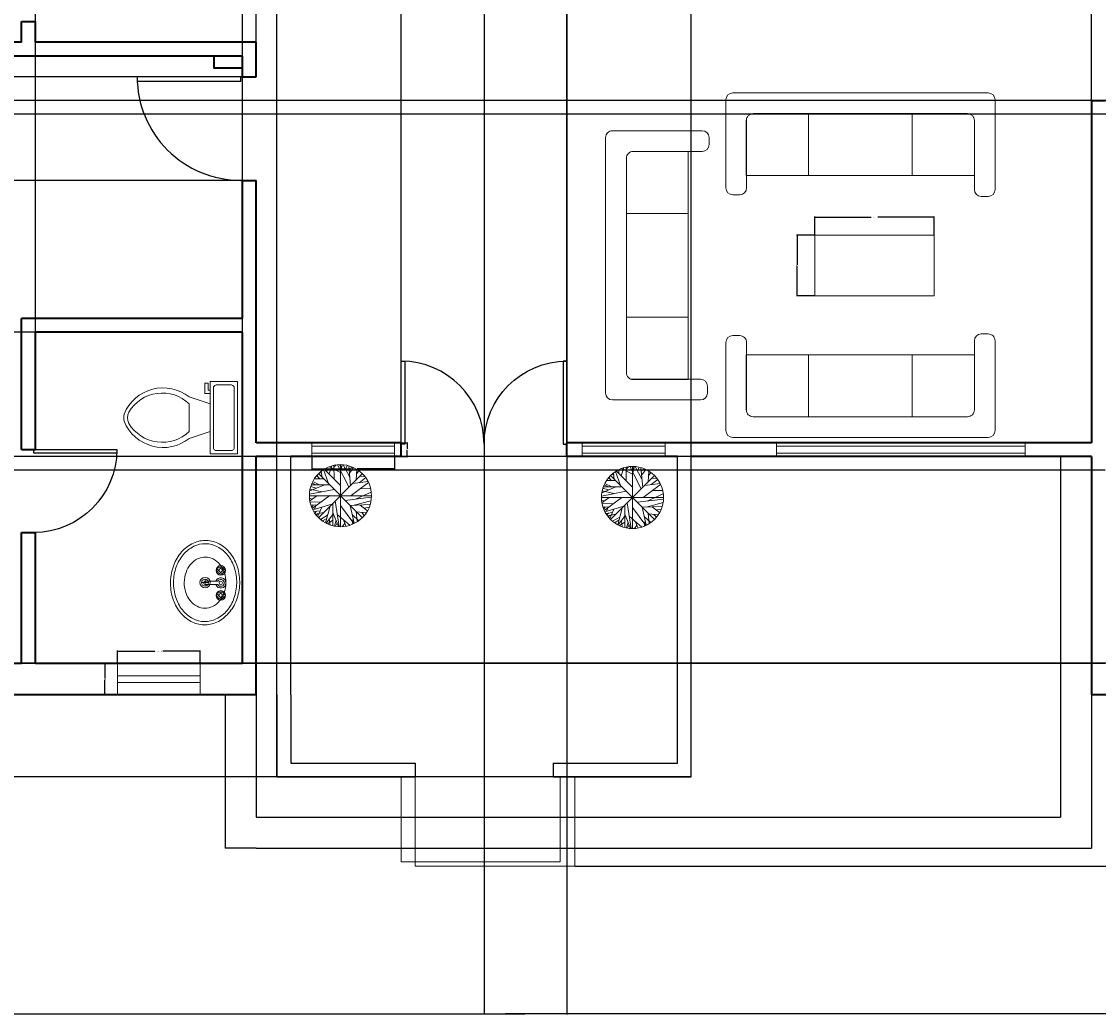
# Model space of a CAD drawing. Units: inches. Extents: x 2024 to 2965, y 1692 to 2308.
# Tile 4 of 8: x 2355 to 2667, y 1692 to 1980. Entities that reach past the tile are written whole.
import ezdxf

# ---------------------------------------------------------------- set-up
doc = ezdxf.new("R2010")
doc.units = ezdxf.units.IN
for name, color, linetype, lineweight in [('A-ANNO-DIMS', 2, 'Continuous', 18), ('A-DOOR', 3, 'Continuous', 25), ('A-FLOR-FIXT', 9, 'Continuous', 18), ('A-FLOR-OTLN', 7, 'Continuous', 25), ('A-FLOR-STRS', 7, 'Continuous', 20), ('A-FURN', 8, 'Continuous', 18), ('A-GLAZ', 4, 'Continuous', 18), ('A-WALL', 7, 'Continuous', 35), ('L-PLNT', 94, 'Continuous', 18)]:
    doc.layers.add(name, color=color, linetype=linetype, lineweight=lineweight)
doc.styles.get("Standard").update_dxf_attribs({"font": 'arial.ttf'})
doc.dimstyles.get("Standard").update_dxf_attribs({"dimtxt": 0.18, "dimasz": 0.18, "dimexe": 0.18, "dimexo": 0.0625, "dimgap": 0.09, "dimtad": 0, "dimtih": 1, "dimtoh": 1, "dimdec": 4, "dimzin": 0, "dimdsep": 46, "dimtxsty": 'Standard', "dimcen": 0.09, "dimadec": 0, "dimazin": 0, "dimtfac": 1, "dimtdec": 4, "dimtofl": 0, "dimtmove": 0, "dimatfit": 3, "dimfxl": 1, "dimtolj": 1, "dimtzin": 0, "dimarcsym": 0})

# ---------------------------------------------------------------- blocks, each defined once
blk = doc.blocks.new('*U7')
for p, q in [((0, 0), (0, -6)), ((40, 0), (40, -6))]:
    blk.add_line(p, q)
blk.add_lwpolyline([(0, 0), (0, 40), (1.75, 40), (1.75, 0)], close=True)
blk.add_arc((0, 0), 40, 0, 90)
blk = doc.blocks.new('*U6')
for p, q in [((0, 0), (0, 6)), ((40, 0), (40, 6))]:
    blk.add_line(p, q)
blk.add_lwpolyline([(0, 0), (0, -40), (1.75, -40), (1.75, 0)], close=True)
blk.add_arc((0, 0), 40, 270, 0)
blk = doc.blocks.new('*U5')
for p, q in [((0, 0), (0, -6)), ((-40, 0), (-40, -6))]:
    blk.add_line(p, q)
blk.add_lwpolyline([(0, 0), (0, 40), (-1.75, 40), (-1.75, 0)], close=True)
blk.add_arc((0, 0), 40, 90, 180)
blk = doc.blocks.new('Toilet - top')
for p, q in [((9.5, -6), (9.5, -2)), ((-10, -8.5), (-8, -8.5)), ((-10, -9.5), (-10, -8.5)), ((-8, -8.5), (-8, -8)), ((-7, -8), (-7, -9.5)), ((-4, -8), (-6, -14)), ((4, -8), (6, -14)), ((-7, -9.5), (-10, -9.5)), ((4, -14), (-4, -14))]:
    blk.add_line(p, q)
blk.add_lwpolyline([(10.5, -8), (10.5, 0), (-10.5, 0), (-10.5, -8)], close=True)
for points in [[(-9.5, -2), (-9.5, -6)], [(8.5, -1), (-8.5, -1)], [(-8.5, -7), (8.5, -7)]]:
    blk.add_lwpolyline(points)
for centre, radius, start, end in [((-8.62, -1.88), 0.884, 81.8699, 188.1301), ((8.62, -1.88), 0.884, 351.8699, 98.1301), ((-8.62, -6.12), 0.884, 171.8699, 278.1301), ((8.62, -6.12), 0.884, 261.8699, 8.1301), ((3.52, -21.58), 12.17, 141.4691, 247.9714), ((4.2, -21.82), 11.33, 136.3677, 238.9468), ((-3.52, -21.58), 12.17, 292.0284, 38.5307), ((-4.2, -21.82), 11.33, 301.053, 43.6321), ((0, -27.88), 4, 245.7318, 294.2682), ((0, -29), 4, 254.8605, 285.1395)]:
    blk.add_arc(centre, radius, start, end)
blk = doc.blocks.new('Sink - Oval top')
for p, q in [((-1, 0), (1, 0)), ((0, 1), (0, -1))]:
    blk.add_line(p, q)
for points in [[(-12.23, 0.39, 0.117634), (-11.46, -3.36, 0.104469), (-8.88, -6.8, 0.090016), (-5.08, -9.07, 0.08192), (-0.32, -10.02, 0.08192), (4.49, -9.38, 0.090016), (8.42, -7.36, 0.104469), (11.22, -4.09, 0.117634), (12.23, -0.39, 0.117634), (11.46, 3.36, 0.104469), (8.88, 6.8, 0.090016), (5.08, 9.07, 0.08192), (0.32, 10.02, 0.08192), (-4.49, 9.38, 0.090016), (-8.42, 7.36, 0.104469), (-11.22, 4.09, 0.117634)], [(-11.29, 0.16, 0.118622), (-10.52, -3.25, 0.104678), (-8.07, -6.36, 0.089562), (-4.54, -8.37, 0.081185), (-0.13, -9.15, 0.081185), (4.3, -8.49, 0.089562), (7.89, -6.58, 0.104678), (10.42, -3.55, 0.118622), (11.29, -0.16, 0.118622), (10.52, 3.25, 0.104678), (8.07, 6.36, 0.089562), (4.54, 8.37, 0.081185), (0.13, 9.15, 0.081185), (-4.3, 8.49, 0.089562), (-7.89, 6.58, 0.104678), (-10.42, 3.55, 0.118622)], [(-7.42, 0.08, 0.118283), (-6.91, -2.17, 0.104607), (-5.29, -4.21, 0.089718), (-2.97, -5.53, 0.081436), (-0.07, -6.04, 0.081436), (2.84, -5.59, 0.089718), (5.2, -4.33, 0.104607), (6.86, -2.32, 0.118283), (7.42, -0.08, 0.118283), (6.91, 2.17, 0.104607), (5.29, 4.21, 0.089718), (2.97, 5.53, 0.081436), (0.07, 6.04, 0.081436), (-2.84, 5.59, 0.089718), (-5.2, 4.33, 0.104607), (-6.86, 2.32, 0.118283)]]:
    blk.add_lwpolyline(points, format="xyb", close=True)
for radius in [1.5, 1]:
    blk.add_circle((0, 0), radius)
blk = doc.blocks.new('Faucet - Bathroom top')
for p, q in [((-4.107, 0.125), (-4.375, 0.125)), ((-3.75, 0.4788), (-3.75, 0.75)), ((-3.5, 0.482), (-3.5, 0.75)), ((-3.1461, 0.125), (-2.875, 0.125)), ((3.143, 0.125), (2.875, 0.125)), ((3.5, 0.4788), (3.5, 0.75)), ((3.75, 0.482), (3.75, 0.75)), ((4.1039, 0.125), (4.375, 0.125)), ((-4.1039, -0.125), (-4.375, -0.125)), ((-3.75, -0.4821), (-3.75, -0.75)), ((-3.5, -0.4789), (-3.5, -0.75)), ((-3.143, -0.125), (-2.875, -0.125)), ((-0.5, -0.8639), (-0.5, -4.5)), ((0.5, -4.5), (0.5, -0.8631)), ((3.1461, -0.125), (2.875, -0.125)), ((3.5, -0.4821), (3.5, -0.75)), ((3.75, -0.4789), (3.75, -0.75)), ((4.107, -0.125), (4.375, -0.125))]:
    blk.add_line(p, q)
for centre, radius in [((-3.625, 0), 1.375), ((-4.625, 0), 0.2795), ((-3.625, 0), 0.5), ((-3.625, 1), 0.2795), ((-2.625, 0), 0.2795), ((0, 0), 0.5), ((3.625, 0), 1.375), ((2.625, 0), 0.2795), ((3.625, 0), 0.5), ((3.625, 1), 0.2795), ((4.625, 0), 0.2795), ((-3.625, -1), 0.2795), ((3.625, -1), 0.2795)]:
    blk.add_circle(centre, radius)
for centre, radius, start, end in [((-3.625, 0), 1, 105.2407, 164.2093), ((-3.625, 0), 1, 16.44125, 74.07887), ((0, 0), 1.5, 289.6514, 250.3603), ((0, 0), 1, 300.3431, 239.7554), ((3.625, 0), 1, 106.12, 164.0884), ((3.625, 0), 1, 16.23422, 73.90469), ((-3.625, 0), 1, 196.2342, 253.9047), ((-3.625, 0), 1, 286.12, 344.0884), ((3.625, 0), 1, 196.4413, 254.0789), ((3.625, 0), 1, 285.2407, 344.2093), ((0, -4.5), 0.5, 180, 0)]:
    blk.add_arc(centre, radius, start, end)
blk = doc.blocks.new('*U19')
for p, q in [((42, 42), (-42, -42)), ((42, -42), (-42, 42)), ((-40.1797, 44.558), (-36.4825, 43.2038)), ((-37.0107, 47.0408), (-35.25, 35.5298)), ((-32.6092, 50.4264), (-23.2782, 23.5674)), ((-31.2008, 51.1035), (-0.2149, 20.1818)), ((-26.4472, 46.5894), (-26.2712, 53.8116)), ((-22.0458, 42.0753), (-16.5881, 57.6486)), ((-21.1656, 55.8436), (-0.0388, 45.0094)), ((-12.5388, 54.9406), (-7.9613, 59.4546)), ((-12.3627, 32.1443), (-12.5388, 58.7776)), ((-5.3205, 59.6806), (16.5105, 16.7963)), ((2.426, 54.9406), (-1.4472, 59.9056)), ((0, 59.9996), (0, -60)), ((0.4894, 48.6208), (3.6584, 59.6806)), ((18.2711, 35.5298), (5.419, 59.6806)), ((9.8203, 51.5549), (12.8133, 58.5516)), ((19.6795, 19.5047), (16.3344, 57.6486)), ((17.0387, 51.1035), (23.2006, 55.1666)), ((17.7429, 43.6552), (25.4894, 54.2636)), ((31.6513, 50.8778), (30.2429, 30.5643)), ((31.1232, 42.5267), (35.8767, 48.1693)), ((-56.0247, 20.859), (-20.8134, 20.859)), ((-54.7923, 24.4702), (-47.75, 21.0847)), ((-53.2078, 27.4044), (-40.1797, 20.859)), ((-49.8627, 32.8214), (-32.7853, 32.8214)), ((-45.8134, 38.2383), (-40.5318, 33.0471)), ((-43.8768, 36.4326), (-44.405, 40.2696)), ((54.3626, 25.3731), (20.9119, 0.3198)), ((23.3767, 23.3417), (53.3063, 27.4044)), ((36.2288, 25.1474), (48.9049, 35.0784)), ((37.1091, 37.1098), (46.6161, 37.5612)), ((-59.7219, 2.8025), (-12.0106, 12.0565)), ((-32.2571, 20.6333), (-59.1937, 9.348)), ((-58.6656, 12.7336), (-35.9543, 7.5424)), ((-57.081, 17.9248), (-47.0458, 14.7649)), ((-54.6162, -24.7335), (-20.2853, 0.0941)), ((29.3626, -6.6771), (59.4682, 7.091)), ((38.5175, 13.4107), (58.2359, 13.6364)), ((-60, 0), (60, 0)), ((-59.7219, -4.8714), (-54.2641, -6.6771)), ((-45.2853, -0.1316), (-59.0177, -10.0627)), ((-58.4895, -12.3197), (-36.4825, -11.6426)), ((-57.081, -18.4138), (-45.2853, -17.9624)), ((-52.6797, -18.188), (-55.4966, -22.0251)), ((-53.2078, -27.442), (-16.7641, -16.6081)), ((-47.2219, -19.3166), (-50.2148, -26.3135)), ((-19.9331, -20.2194), (-28.5599, -52.721)), ((-14.8275, -15.0282), (-14.6515, -57.6865)), ((-10.074, -10.0627), (-2.5036, -59.7178)), ((-0.0388, -19.0909), (25.8415, -53.8495)), ((9.2922, -9.1598), (59.6443, -2.8401)), ((18.6232, -18.6394), (26.7218, -53.3981)), ((18.7992, -18.6394), (57.3556, -17.2853)), ((26.3697, -18.4138), (58.9401, -9.8369)), ((38.1654, -18.188), (52.426, -29.0219)), ((-38.9472, -29.0219), (-51.4472, -30.6018)), ((-46.5177, -30.1504), (-49.5106, -33.536)), ((-32.4331, -32.4075), (-48.1021, -35.5674)), ((-43.7008, -34.6645), (-46.6937, -37.373)), ((-35.9543, -22.4765), (-44.0529, -40.5329)), ((-24.6867, -37.8244), (-38.7712, -45.7241)), ((-14.6515, -36.2445), (-27.6797, -52.9467)), ((-14.6515, -32.1818), (-3.912, -59.4922)), ((-6.2008, -36.2445), (17.919, -57.0094)), ((22.8485, -36.4702), (35.3485, -48.4326)), ((30.419, -30.1504), (32.3556, -50.0125)), ((31.4753, -31.279), (49.6091, -33.3103)), ((41.5105, -32.6332), (46.088, -38.0501)), ((45.9119, -24.0564), (55.595, -22.2508)), ((-26.2712, -43.9185), (-34.7219, -48.6583)), ((-14.6515, -47.3041), (-25.0388, -54.3009)), ((-21.5177, -45.4984), (-19.9331, -56.1065)), ((-8.4895, -47.5298), (-11.4825, -58.5893)), ((-6.3768, -52.721), (-9.3698, -58.815)), ((8.4119, -53.1724), (3.8344, -59.4922)), ((5.9471, -46.6269), (10.5246, -58.5893)), ((24.7852, -44.8213), (23.0246, -54.978))]:
    blk.add_line(p, q)
blk.add_circle((0, 0), 60)
blk = doc.blocks.new('WIN-24-D9')
for p, q in [((0, 5.5), (24, 5.5)), ((0, 3.5), (24, 3.5))]:
    blk.add_line(p, q)
for points in [[(0, 0), (0, 9)], [(24, 9), (24, 0)]]:
    blk.add_lwpolyline(points)
blk = doc.blocks.new('WIN-72-D4')
for p, q in [((0, 3), (72, 3)), ((0, 1), (72, 1))]:
    blk.add_line(p, q)
for points in [[(0, 0), (0, 4)], [(72, 4), (72, 0)]]:
    blk.add_lwpolyline(points)
blk = doc.blocks.new('WIN-24-D4')
for p, q in [((0, 3), (24, 3)), ((0, 1), (24, 1))]:
    blk.add_line(p, q)
for points in [[(0, 0), (0, 4)], [(24, 4), (24, 0)]]:
    blk.add_lwpolyline(points)
blk = doc.blocks.new('SOFA-78')
for p, q in [((2, 30), (76, 30)), ((0, 2.5), (0, 28)), ((78, 28), (78, 2)), ((6, 22.6), (6, 2.5)), ((70, 24), (7.91, 24)), ((72, 2), (72, 22)), ((4, 0.5), (2, 0.5)), ((76, 0), (74, 0))]:
    blk.add_line(p, q)
for points in [[(23.94, 24), (7.91, 24, 0.414214), (5.91, 22), (5.91, 6.04), (23.94, 6.04)], [(70, 24), (53.97, 24), (53.97, 6.04), (72, 6.04), (72, 22, 0.414214)]]:
    blk.add_lwpolyline(points, format="xyb", close=True)
for points in [[(35.94, 24), (17.9, 24)], [(35.94, 6.04), (53.97, 6.04), (53.97, 24), (35.94, 24)], [(17.9, 6.04), (35.94, 6.04)]]:
    blk.add_lwpolyline(points)
for centre, start, end in [((2, 28), 90, 180), ((76, 28), 0, 90), ((70, 22), 0, 90), ((2, 2.5), 180, 270), ((4, 2.5), 270, 0), ((74, 2), 180, 270), ((76, 2), 270, 0)]:
    blk.add_arc(centre, 2, start, end)
blk = doc.blocks.new('COFFEE-TABLE')
blk.add_lwpolyline([(0, 17.56), (34.53, 17.56), (34.53, 0), (0, 0)], close=True)
blk = doc.blocks.new('*D29')
at = {"layer": 'A-ANNO-DIMS', "color": 0, "lineweight": -2, "transparency": 16777216}
for p, q in [((2382.68, 1793.84), (2382.68, 1797.55)), ((2382.86, 1797.37), (2393.56, 1797.37)), ((2406.5, 1797.37), (2395.8, 1797.37)), ((2406.68, 1793.84), (2406.68, 1797.55))]:
    blk.add_line(p, q, dxfattribs=at)
at = {"layer": 'A-ANNO-DIMS', "color": 0, "transparency": 16777216}
for points in [[(2382.86, 1797.4), (2382.86, 1797.34), (2382.68, 1797.37)], [(2406.5, 1797.4), (2406.5, 1797.34), (2406.68, 1797.37)]]:
    blk.add_solid(points, dxfattribs=at)
at = {"layer": 'Defpoints', "color": 0, "transparency": 16777216}
for p in [(2382.68, 1797.37), (2382.68, 1793.77), (2406.68, 1793.77)]:
    blk.add_point(p, dxfattribs=at)
at = {"layer": 'A-ANNO-DIMS', "color": 0, "transparency": 16777216, "insert": (2394.68, 1797.37), "char_height": 0.18, "attachment_point": 5}
blk.add_mtext('\\A1;WINDOW 24 TYP.', dxfattribs=at)
blk = doc.blocks.new('*D30')
at = {"layer": 'A-ANNO-DIMS', "color": 0, "lineweight": -2, "transparency": 16777216}
for p, q in [((2382.61, 1793.77), (2378.9, 1793.77)), ((2379.08, 1793.59), (2379.08, 1789.46)), ((2379.08, 1784.95), (2379.08, 1789.09)), ((2382.61, 1784.77), (2378.9, 1784.77))]:
    blk.add_line(p, q, dxfattribs=at)
at = {"layer": 'A-ANNO-DIMS', "color": 0, "transparency": 16777216}
for points in [[(2379.05, 1793.59), (2379.11, 1793.59), (2379.08, 1793.77)], [(2379.05, 1784.95), (2379.11, 1784.95), (2379.08, 1784.77)]]:
    blk.add_solid(points, dxfattribs=at)
at = {"layer": 'Defpoints', "color": 0, "transparency": 16777216}
for p in [(2382.68, 1793.77), (2379.08, 1784.77), (2382.68, 1784.77)]:
    blk.add_point(p, dxfattribs=at)
at = {"layer": 'A-ANNO-DIMS', "color": 0, "transparency": 16777216, "insert": (2379.08, 1789.27), "char_height": 0.18, "attachment_point": 5}
blk.add_mtext('\\A1;9 TYP.', dxfattribs=at)
blk = doc.blocks.new('*D37')
at = {"layer": 'A-ANNO-DIMS', "color": 0, "lineweight": -2, "transparency": 16777216}
for p, q in [((2439, 1853.71), (2439, 1849.99)), ((2463, 1853.71), (2463, 1849.99)), ((2439.18, 1850.17), (2449.88, 1850.17)), ((2462.82, 1850.17), (2452.11, 1850.17))]:
    blk.add_line(p, q, dxfattribs=at)
at = {"layer": 'A-ANNO-DIMS', "color": 0, "transparency": 16777216}
for points in [[(2439.18, 1850.2), (2439.18, 1850.14), (2439, 1850.17)], [(2462.82, 1850.2), (2462.82, 1850.14), (2463, 1850.17)]]:
    blk.add_solid(points, dxfattribs=at)
at = {"layer": 'Defpoints', "color": 0, "transparency": 16777216}
for p in [(2439, 1853.77), (2463, 1853.77), (2463, 1850.17)]:
    blk.add_point(p, dxfattribs=at)
at = {"layer": 'A-ANNO-DIMS', "color": 0, "transparency": 16777216, "insert": (2451, 1850.17), "char_height": 0.18, "attachment_point": 5}
blk.add_mtext('\\A1;WINDOW 24 TYP.', dxfattribs=at)
blk = doc.blocks.new('*D38')
at = {"layer": 'A-ANNO-DIMS', "color": 0, "lineweight": -2, "transparency": 16777216}
for p, q in [((2463.06, 1857.77), (2466.78, 1857.77)), ((2466.6, 1857.59), (2466.6, 1855.95)), ((2463.06, 1853.77), (2466.78, 1853.77)), ((2466.6, 1853.95), (2466.6, 1855.59))]:
    blk.add_line(p, q, dxfattribs=at)
at = {"layer": 'A-ANNO-DIMS', "color": 0, "transparency": 16777216}
for points in [[(2466.57, 1857.59), (2466.63, 1857.59), (2466.6, 1857.77)], [(2466.57, 1853.95), (2466.63, 1853.95), (2466.6, 1853.77)]]:
    blk.add_solid(points, dxfattribs=at)
at = {"layer": 'Defpoints', "color": 0, "transparency": 16777216}
for p in [(2463, 1857.77), (2466.6, 1857.77), (2463, 1853.77)]:
    blk.add_point(p, dxfattribs=at)
at = {"layer": 'A-ANNO-DIMS', "color": 0, "transparency": 16777216, "insert": (2466.6, 1855.77), "char_height": 0.18, "attachment_point": 5}
blk.add_mtext('\\A1;4 TYP.', dxfattribs=at)
blk = doc.blocks.new('*D41')
at = {"layer": 'A-ANNO-DIMS', "color": 0, "lineweight": -2, "transparency": 16777216}
for p, q in [((2584.78, 1917.99), (2584.78, 1923.28)), ((2584.96, 1923.1), (2601.08, 1923.1)), ((2619.13, 1923.1), (2603.01, 1923.1)), ((2619.31, 1917.99), (2619.31, 1923.28))]:
    blk.add_line(p, q, dxfattribs=at)
at = {"layer": 'A-ANNO-DIMS', "color": 0, "transparency": 16777216}
for points in [[(2584.96, 1923.13), (2584.96, 1923.07), (2584.78, 1923.1)], [(2619.13, 1923.13), (2619.13, 1923.07), (2619.31, 1923.1)]]:
    blk.add_solid(points, dxfattribs=at)
at = {"layer": 'Defpoints', "color": 0, "transparency": 16777216}
for p in [(2619.31, 1923.1), (2584.78, 1917.92), (2619.31, 1917.92)]:
    blk.add_point(p, dxfattribs=at)
at = {"layer": 'A-ANNO-DIMS', "color": 0, "transparency": 16777216, "insert": (2602.04, 1923.1), "char_height": 0.18, "attachment_point": 5}
blk.add_mtext('\\A1;TABLE 35 TYP.', dxfattribs=at)
blk = doc.blocks.new('*D42')
at = {"layer": 'A-ANNO-DIMS', "color": 0, "lineweight": -2, "transparency": 16777216}
for p, q in [((2584.72, 1917.92), (2579.42, 1917.92)), ((2579.6, 1917.74), (2579.6, 1909.33)), ((2579.6, 1900.54), (2579.6, 1908.96)), ((2584.72, 1900.36), (2579.42, 1900.36))]:
    blk.add_line(p, q, dxfattribs=at)
at = {"layer": 'A-ANNO-DIMS', "color": 0, "transparency": 16777216}
for points in [[(2579.57, 1917.74), (2579.63, 1917.74), (2579.6, 1917.92)], [(2579.57, 1900.54), (2579.63, 1900.54), (2579.6, 1900.36)]]:
    blk.add_solid(points, dxfattribs=at)
at = {"layer": 'Defpoints', "color": 0, "transparency": 16777216}
for p in [(2579.6, 1917.92), (2584.78, 1917.92), (2584.78, 1900.36)]:
    blk.add_point(p, dxfattribs=at)
at = {"layer": 'A-ANNO-DIMS', "color": 0, "transparency": 16777216, "insert": (2579.6, 1909.14), "char_height": 0.18, "attachment_point": 5}
blk.add_mtext('\\A1;18 TYP.', dxfattribs=at)
blk = doc.blocks.new('*D75')
at = {"layer": 'A-ANNO-DIMS', "color": 0, "lineweight": -2, "transparency": 16777216}
for p, q in [((2922.02, 1952.85), (2922.02, 1692.14)), ((2067.46, 1932.29), (2067.46, 1692.14)), ((2067.64, 1692.32), (2494.35, 1692.32)), ((2921.84, 1692.32), (2495.13, 1692.32))]:
    blk.add_line(p, q, dxfattribs=at)
at = {"layer": 'A-ANNO-DIMS', "color": 0, "transparency": 16777216}
for points in [[(2067.64, 1692.35), (2067.64, 1692.29), (2067.46, 1692.32)], [(2921.84, 1692.35), (2921.84, 1692.29), (2922.02, 1692.32)]]:
    blk.add_solid(points, dxfattribs=at)
at = {"layer": 'Defpoints', "color": 0, "transparency": 16777216}
for p in [(2922.02, 1952.91), (2067.46, 1932.35), (2922.02, 1692.32)]:
    blk.add_point(p, dxfattribs=at)
at = {"layer": 'A-ANNO-DIMS', "color": 0, "transparency": 16777216, "insert": (2494.74, 1692.32), "char_height": 0.18, "attachment_point": 5}
blk.add_mtext('\\A1;854.6', dxfattribs=at)
blk = doc.blocks.new('*D76')
at = {"layer": 'A-ANNO-DIMS', "color": 0, "lineweight": -2, "transparency": 16777216}
for p, q in [((2718.97, 2264.77), (2964.97, 2264.77)), ((2964.79, 2264.59), (2964.79, 2000.12)), ((2964.79, 1735.28), (2964.79, 1999.75)), ((2515.28, 1735.1), (2964.97, 1735.1))]:
    blk.add_line(p, q, dxfattribs=at)
at = {"layer": 'A-ANNO-DIMS', "color": 0, "transparency": 16777216}
for points in [[(2964.76, 2264.59), (2964.82, 2264.59), (2964.79, 2264.77)], [(2964.76, 1735.28), (2964.82, 1735.28), (2964.79, 1735.1)]]:
    blk.add_solid(points, dxfattribs=at)
at = {"layer": 'Defpoints', "color": 0, "transparency": 16777216}
for p in [(2718.91, 2264.77), (2515.22, 1735.1), (2964.79, 1735.1)]:
    blk.add_point(p, dxfattribs=at)
at = {"layer": 'A-ANNO-DIMS', "color": 0, "transparency": 16777216, "insert": (2964.79, 1999.94), "char_height": 0.18, "attachment_point": 5}
blk.add_mtext('\\A1;529.7', dxfattribs=at)
blk = doc.blocks.new('*D93')
at = {"layer": 'A-ANNO-DIMS', "color": 0, "lineweight": -2, "transparency": 16777216}
for p, q in [((2187.46, 1932.41), (2187.46, 2307.73)), ((2187.64, 2307.55), (2302.72, 2307.55)), ((2418.73, 2307.55), (2303.65, 2307.55)), ((2418.91, 1933.84), (2418.91, 2307.73))]:
    blk.add_line(p, q, dxfattribs=at)
at = {"layer": 'A-ANNO-DIMS', "color": 0, "transparency": 16777216}
for points in [[(2187.64, 2307.58), (2187.64, 2307.52), (2187.46, 2307.55)], [(2418.73, 2307.58), (2418.73, 2307.52), (2418.91, 2307.55)]]:
    blk.add_solid(points, dxfattribs=at)
at = {"layer": 'Defpoints', "color": 0, "transparency": 16777216}
for p in [(2418.91, 2307.55), (2187.46, 1932.35), (2418.91, 1933.77)]:
    blk.add_point(p, dxfattribs=at)
at = {"layer": 'A-ANNO-DIMS', "color": 0, "transparency": 16777216, "insert": (2303.18, 2307.55), "char_height": 0.18, "attachment_point": 5}
blk.add_mtext('\\A1;231.45', dxfattribs=at)
blk = doc.blocks.new('*D96')
at = {"layer": 'A-ANNO-DIMS', "color": 0, "lineweight": -2, "transparency": 16777216}
for p, q in [((2358.91, 1889.84), (2358.91, 2307.73)), ((2359.09, 2307.55), (2388.69, 2307.55)), ((2418.73, 2307.55), (2389.13, 2307.55)), ((2418.91, 1889.84), (2418.91, 2307.73))]:
    blk.add_line(p, q, dxfattribs=at)
at = {"layer": 'A-ANNO-DIMS', "color": 0, "transparency": 16777216}
for points in [[(2359.09, 2307.58), (2359.09, 2307.52), (2358.91, 2307.55)], [(2418.73, 2307.58), (2418.73, 2307.52), (2418.91, 2307.55)]]:
    blk.add_solid(points, dxfattribs=at)
at = {"layer": 'Defpoints', "color": 0, "transparency": 16777216}
for p in [(2418.91, 2307.55), (2358.91, 1889.77), (2418.91, 1889.77)]:
    blk.add_point(p, dxfattribs=at)
at = {"layer": 'A-ANNO-DIMS', "color": 0, "transparency": 16777216, "insert": (2388.91, 2307.55), "char_height": 0.18, "attachment_point": 5}
blk.add_mtext('\\A1;60', dxfattribs=at)
blk = doc.blocks.new('*D97')
at = {"layer": 'A-ANNO-DIMS', "color": 0, "lineweight": -2, "transparency": 16777216}
for p, q in [((2358.84, 1889.77), (2024.5, 1889.77)), ((2024.68, 1889.59), (2024.68, 1841.96)), ((2024.68, 1793.95), (2024.68, 1841.59)), ((2358.84, 1793.77), (2024.5, 1793.77))]:
    blk.add_line(p, q, dxfattribs=at)
at = {"layer": 'A-ANNO-DIMS', "color": 0, "transparency": 16777216}
for points in [[(2024.65, 1889.59), (2024.71, 1889.59), (2024.68, 1889.77)], [(2024.65, 1793.95), (2024.71, 1793.95), (2024.68, 1793.77)]]:
    blk.add_solid(points, dxfattribs=at)
at = {"layer": 'Defpoints', "color": 0, "transparency": 16777216}
for p in [(2358.91, 1889.77), (2024.68, 1793.77), (2358.91, 1793.77)]:
    blk.add_point(p, dxfattribs=at)
at = {"layer": 'A-ANNO-DIMS', "color": 0, "transparency": 16777216, "insert": (2024.68, 1841.77), "char_height": 0.18, "attachment_point": 5}
blk.add_mtext('\\A1;96', dxfattribs=at)
blk = doc.blocks.new('*D98')
at = {"layer": 'A-ANNO-DIMS', "color": 0, "lineweight": -2, "transparency": 16777216}
for p, q in [((2422.91, 1973.84), (2422.91, 2307.73)), ((2423.09, 2307.55), (2543.62, 2307.55)), ((2664.73, 2307.55), (2544.2, 2307.55)), ((2664.91, 1956.85), (2664.91, 2307.73))]:
    blk.add_line(p, q, dxfattribs=at)
at = {"layer": 'A-ANNO-DIMS', "color": 0, "transparency": 16777216}
for points in [[(2423.09, 2307.58), (2423.09, 2307.52), (2422.91, 2307.55)], [(2664.73, 2307.58), (2664.73, 2307.52), (2664.91, 2307.55)]]:
    blk.add_solid(points, dxfattribs=at)
at = {"layer": 'Defpoints', "color": 0, "transparency": 16777216}
for p in [(2664.91, 2307.55), (2422.91, 1973.77), (2664.91, 1956.79)]:
    blk.add_point(p, dxfattribs=at)
at = {"layer": 'A-ANNO-DIMS', "color": 0, "transparency": 16777216, "insert": (2543.91, 2307.55), "char_height": 0.18, "attachment_point": 5}
blk.add_mtext('\\A1;242', dxfattribs=at)
blk = doc.blocks.new('*D101')
at = {"layer": 'A-ANNO-DIMS', "color": 0, "lineweight": -2, "transparency": 16777216}
for p, q in [((2917.96, 2113.77), (2024.5, 2113.77)), ((2024.68, 2113.59), (2024.68, 2035.52)), ((2024.68, 1957.09), (2024.68, 2035.16)), ((2917.96, 1956.91), (2024.5, 1956.91))]:
    blk.add_line(p, q, dxfattribs=at)
at = {"layer": 'A-ANNO-DIMS', "color": 0, "transparency": 16777216}
for points in [[(2024.65, 2113.59), (2024.71, 2113.59), (2024.68, 2113.77)], [(2024.65, 1957.09), (2024.71, 1957.09), (2024.68, 1956.91)]]:
    blk.add_solid(points, dxfattribs=at)
at = {"layer": 'Defpoints', "color": 0, "transparency": 16777216}
for p in [(2024.68, 2113.77), (2918.02, 2113.77), (2918.02, 1956.91)]:
    blk.add_point(p, dxfattribs=at)
at = {"layer": 'A-ANNO-DIMS', "color": 0, "transparency": 16777216, "insert": (2024.68, 2035.34), "char_height": 0.18, "attachment_point": 5}
blk.add_mtext('\\A1;156.87', dxfattribs=at)
blk = doc.blocks.new('*D102')
at = {"layer": 'A-ANNO-DIMS', "color": 0, "lineweight": -2, "transparency": 16777216}
for p, q in [((2830.9, 1952.91), (2024.5, 1952.91)), ((2024.68, 1952.73), (2024.68, 1873.58)), ((2024.68, 1794.07), (2024.68, 1873.22)), ((2830.9, 1793.89), (2024.5, 1793.89))]:
    blk.add_line(p, q, dxfattribs=at)
at = {"layer": 'A-ANNO-DIMS', "color": 0, "transparency": 16777216}
for points in [[(2024.65, 1952.73), (2024.71, 1952.73), (2024.68, 1952.91)], [(2024.65, 1794.07), (2024.71, 1794.07), (2024.68, 1793.89)]]:
    blk.add_solid(points, dxfattribs=at)
at = {"layer": 'Defpoints', "color": 0, "transparency": 16777216}
for p in [(2830.96, 1952.91), (2024.68, 1793.89), (2830.96, 1793.89)]:
    blk.add_point(p, dxfattribs=at)
at = {"layer": 'A-ANNO-DIMS', "color": 0, "transparency": 16777216, "insert": (2024.68, 1873.4), "char_height": 0.18, "attachment_point": 5}
blk.add_mtext('\\A1;159', dxfattribs=at)
blk = doc.blocks.new('*D103')
at = {"layer": 'A-ANNO-DIMS', "color": 0, "lineweight": -2, "transparency": 16777216}
for p, q in [((2464.91, 1881.44), (2464.91, 2307.73)), ((2465.09, 2307.55), (2488.68, 2307.55)), ((2512.73, 2307.55), (2489.13, 2307.55)), ((2512.91, 1881.44), (2512.91, 2307.73))]:
    blk.add_line(p, q, dxfattribs=at)
at = {"layer": 'A-ANNO-DIMS', "color": 0, "transparency": 16777216}
for points in [[(2465.09, 2307.58), (2465.09, 2307.52), (2464.91, 2307.55)], [(2512.73, 2307.58), (2512.73, 2307.52), (2512.91, 2307.55)]]:
    blk.add_solid(points, dxfattribs=at)
at = {"layer": 'Defpoints', "color": 0, "transparency": 16777216}
for p in [(2512.91, 2307.55), (2464.91, 1881.37), (2512.91, 1881.37)]:
    blk.add_point(p, dxfattribs=at)
at = {"layer": 'A-ANNO-DIMS', "color": 0, "transparency": 16777216, "insert": (2488.91, 2307.55), "char_height": 0.18, "attachment_point": 5}
blk.add_mtext('\\A1;48', dxfattribs=at)
blk = doc.blocks.new('*D104')
at = {"layer": 'A-ANNO-DIMS', "color": 0, "lineweight": -2, "transparency": 16777216}
for p, q in [((2418.84, 1963.77), (2024.5, 1963.77)), ((2024.68, 1963.59), (2024.68, 1948.96)), ((2024.68, 1933.95), (2024.68, 1948.59)), ((2418.84, 1933.77), (2024.5, 1933.77))]:
    blk.add_line(p, q, dxfattribs=at)
at = {"layer": 'A-ANNO-DIMS', "color": 0, "transparency": 16777216}
for points in [[(2024.65, 1963.59), (2024.71, 1963.59), (2024.68, 1963.77)], [(2024.65, 1933.95), (2024.71, 1933.95), (2024.68, 1933.77)]]:
    blk.add_solid(points, dxfattribs=at)
at = {"layer": 'Defpoints', "color": 0, "transparency": 16777216}
for p in [(2418.91, 1963.77), (2024.68, 1933.77), (2418.91, 1933.77)]:
    blk.add_point(p, dxfattribs=at)
at = {"layer": 'A-ANNO-DIMS', "color": 0, "transparency": 16777216, "insert": (2024.68, 1948.77), "char_height": 0.18, "attachment_point": 5}
blk.add_mtext('\\A1;30', dxfattribs=at)
blk = doc.blocks.new('*D109')
at = {"layer": 'A-ANNO-DIMS', "color": 0, "lineweight": -2, "transparency": 16777216}
for p, q in [((2488.89, 2214.47), (2488.89, 1692.14)), ((2512.89, 2214.58), (2512.89, 1692.14)), ((2489.07, 1692.32), (2500.67, 1692.32)), ((2512.71, 1692.32), (2501.11, 1692.32))]:
    blk.add_line(p, q, dxfattribs=at)
at = {"layer": 'A-ANNO-DIMS', "color": 0, "transparency": 16777216}
for points in [[(2489.07, 1692.35), (2489.07, 1692.29), (2488.89, 1692.32)], [(2512.71, 1692.35), (2512.71, 1692.29), (2512.89, 1692.32)]]:
    blk.add_solid(points, dxfattribs=at)
at = {"layer": 'Defpoints', "color": 0, "transparency": 16777216}
for p in [(2488.89, 2214.53), (2512.89, 2214.64), (2512.89, 1692.32)]:
    blk.add_point(p, dxfattribs=at)
at = {"layer": 'A-ANNO-DIMS', "color": 0, "transparency": 16777216, "insert": (2500.89, 1692.32), "char_height": 0.18, "attachment_point": 5}
blk.add_mtext('\\A1;24', dxfattribs=at)
blk = doc.blocks.new('*D111')
at = {"layer": 'A-ANNO-DIMS', "color": 0, "lineweight": -2, "transparency": 16777216}
for p, q in [((2668.84, 1849.79), (2024.5, 1849.79)), ((2024.68, 1849.61), (2024.68, 1821.96)), ((2024.68, 1793.95), (2024.68, 1821.6)), ((2668.84, 1793.77), (2024.5, 1793.77))]:
    blk.add_line(p, q, dxfattribs=at)
at = {"layer": 'A-ANNO-DIMS', "color": 0, "transparency": 16777216}
for points in [[(2024.65, 1849.61), (2024.71, 1849.61), (2024.68, 1849.79)], [(2024.65, 1793.95), (2024.71, 1793.95), (2024.68, 1793.77)]]:
    blk.add_solid(points, dxfattribs=at)
at = {"layer": 'Defpoints', "color": 0, "transparency": 16777216}
for p in [(2024.68, 1849.79), (2668.91, 1849.79), (2668.91, 1793.77)]:
    blk.add_point(p, dxfattribs=at)
at = {"layer": 'A-ANNO-DIMS', "color": 0, "transparency": 16777216, "insert": (2024.68, 1821.78), "char_height": 0.18, "attachment_point": 5}
blk.add_mtext('\\A1;56.01', dxfattribs=at)
blk = doc.blocks.new('*D114')
at = {"layer": 'A-ANNO-DIMS', "color": 0, "lineweight": -2, "transparency": 16777216}
for p, q in [((2428.91, 1761.01), (2428.91, 2307.73)), ((2429.09, 2307.55), (2488.63, 2307.55)), ((2548.73, 2307.55), (2489.19, 2307.55)), ((2548.91, 1761.01), (2548.91, 2307.73))]:
    blk.add_line(p, q, dxfattribs=at)
at = {"layer": 'A-ANNO-DIMS', "color": 0, "transparency": 16777216}
for points in [[(2429.09, 2307.58), (2429.09, 2307.52), (2428.91, 2307.55)], [(2548.73, 2307.58), (2548.73, 2307.52), (2548.91, 2307.55)]]:
    blk.add_solid(points, dxfattribs=at)
at = {"layer": 'Defpoints', "color": 0, "transparency": 16777216}
for p in [(2548.91, 2307.55), (2428.91, 1760.95), (2548.91, 1760.95)]:
    blk.add_point(p, dxfattribs=at)
at = {"layer": 'A-ANNO-DIMS', "color": 0, "transparency": 16777216, "insert": (2488.91, 2307.55), "char_height": 0.18, "attachment_point": 5}
blk.add_mtext('\\A1;120', dxfattribs=at)
blk = doc.blocks.new('*D115')
at = {"layer": 'A-ANNO-DIMS', "color": 0, "lineweight": -2, "transparency": 16777216}
for p, q in [((2548.84, 1853.77), (2024.5, 1853.77)), ((2024.68, 1853.59), (2024.68, 1807.54)), ((2024.68, 1761.13), (2024.68, 1807.18)), ((2548.84, 1760.95), (2024.5, 1760.95))]:
    blk.add_line(p, q, dxfattribs=at)
at = {"layer": 'A-ANNO-DIMS', "color": 0, "transparency": 16777216}
for points in [[(2024.65, 1853.59), (2024.71, 1853.59), (2024.68, 1853.77)], [(2024.65, 1761.13), (2024.71, 1761.13), (2024.68, 1760.95)]]:
    blk.add_solid(points, dxfattribs=at)
at = {"layer": 'Defpoints', "color": 0, "transparency": 16777216}
for p in [(2024.68, 1853.77), (2548.91, 1853.77), (2548.91, 1760.95)]:
    blk.add_point(p, dxfattribs=at)
at = {"layer": 'A-ANNO-DIMS', "color": 0, "transparency": 16777216, "insert": (2024.68, 1807.36), "char_height": 0.18, "attachment_point": 5}
blk.add_mtext('\\A1;92.82', dxfattribs=at)

msp = doc.modelspace()

# ---------------------------------------------------------------- linework, layer by layer
at = {"layer": 'A-FLOR-OTLN'}
for p, q in [((2428.9061, 1784.7736), (2428.9061, 1853.7736)), ((2432.9061, 1784.7736), (2432.9061, 1853.7736)), ((2544.9061, 1764.9504), (2544.9061, 1853.7736)), ((2548.9061, 1760.9504), (2548.9061, 1853.7736)), ((2655.9061, 1853.7736), (2655.9061, 1784.7736)), ((2413.9061, 1784.7736), (2413.9061, 1749.2678)), ((2422.9061, 1784.7736), (2422.9061, 1749.2678)), ((2428.9061, 1784.7736), (2428.9061, 1760.9504)), ((2432.9061, 1784.7736), (2432.9061, 1764.9504)), ((2655.9061, 1784.7736), (2655.9061, 1749.2678)), ((2664.9061, 1784.7736), (2664.9061, 1740.2678)), ((2432.9061, 1764.9504), (2468.9061, 1764.9504)), ((2468.9061, 1764.9504), (2468.9061, 1760.9504)), ((2508.9061, 1764.9504), (2508.9061, 1760.9504)), ((2508.9061, 1764.9504), (2544.9061, 1764.9504)), ((2428.9061, 1760.9504), (2468.9061, 1760.9504)), ((2508.9061, 1760.9504), (2548.9061, 1760.9504)), ((2413.9061, 1749.2678), (2413.9061, 1740.2678)), ((2422.9061, 1749.2678), (2655.9061, 1749.2678)), ((2422.9061, 1740.2678), (2413.9061, 1740.2678)), ((2422.9061, 1740.2678), (2653.4158, 1740.2678)), ((2653.4158, 1740.2678), (2664.9061, 1740.2678))]:
    msp.add_line(p, q, dxfattribs=at)
at = {"layer": 'A-FLOR-STRS'}
for points in [[(2464.9278, 1760.9504), (2510.9128, 1760.9504), (2510.9128, 1736.3585), (2464.9278, 1736.3585)], [(2468.9061, 1760.9504), (2515.2195, 1760.9504), (2515.2195, 1735.0986), (2468.9061, 1735.0986)]]:
    msp.add_lwpolyline(points, close=True, dxfattribs=at)
at = {"layer": 'A-WALL'}
for p, q in [((2354.9061, 1973.7736), (2354.9061, 1979.7736)), ((2354.9061, 1979.7736), (2358.9061, 1979.7736)), ((2358.9061, 1973.7736), (2358.9061, 1979.7736)), ((2354.9061, 1973.7736), (2187.4594, 1973.7736)), ((2422.9061, 1973.7736), (2358.9061, 1973.7736)), ((2422.9061, 1963.7736), (2422.9061, 1973.7736)), ((2354.9061, 1969.7736), (2187.4594, 1969.7736)), ((2418.9061, 1969.7736), (2354.9061, 1969.7736)), ((2418.9061, 1963.7736), (2418.9061, 1969.7736)), ((2418.9061, 1963.7736), (2422.9061, 1963.7736)), ((2664.9061, 1956.7881), (2664.9061, 1857.7736)), ((2668.9061, 1956.7881), (2664.9061, 1956.7881)), ((2418.9061, 1933.7736), (2422.9061, 1933.7736)), ((2418.9061, 1893.7736), (2418.9061, 1933.7736)), ((2422.9061, 1857.7736), (2422.9061, 1933.7736)), ((2418.9061, 1893.7736), (2354.9061, 1893.7736)), ((2354.9061, 1855.7736), (2354.9061, 1893.7736)), ((2418.9061, 1889.7736), (2358.9061, 1889.7736)), ((2358.9061, 1855.7736), (2358.9061, 1889.7736)), ((2418.9061, 1793.7736), (2418.9061, 1889.7736)), ((2464.9061, 1857.7736), (2422.9061, 1857.7736)), ((2464.9061, 1853.7736), (2464.9061, 1857.7736)), ((2664.9061, 1857.7736), (2512.9061, 1857.7736)), ((2512.9061, 1853.7736), (2512.9061, 1857.7736)), ((2354.9061, 1855.7736), (2358.9061, 1855.7736)), ((2422.9061, 1784.7736), (2422.9061, 1853.7736)), ((2428.9061, 1853.7736), (2422.9061, 1853.7736)), ((2464.9061, 1853.7736), (2432.9061, 1853.7736)), ((2544.9061, 1853.7736), (2512.9061, 1853.7736)), ((2664.9061, 1853.7736), (2548.9061, 1853.7736)), ((2664.9061, 1853.7736), (2664.9061, 1784.7736)), ((2354.9061, 1793.7736), (2354.9061, 1831.7736)), ((2354.9061, 1831.7736), (2358.9061, 1831.7736)), ((2358.9061, 1793.7736), (2358.9061, 1831.7736)), ((2354.9061, 1793.7736), (2170.9061, 1793.7736)), ((2418.9061, 1793.7736), (2358.9061, 1793.7736))]:
    msp.add_line(p, q, dxfattribs=at)
msp.add_lwpolyline([(2418.9061, 1969.7736), (2410.6411, 1969.7736), (2410.6411, 1966.3665), (2418.9061, 1966.3665)], close=True, dxfattribs=at)
for points in [[(2422.9061, 1784.7736), (2161.9061, 1784.7736), (2161.9061, 1932.352)], [(2761.9061, 1784.7736), (2664.9061, 1784.7736)]]:
    msp.add_lwpolyline(points, dxfattribs=at)

# ---------------------------------------------------------------- block references
at = {"layer": 'A-DOOR', "rotation": 270}
for name, p, xscale, yscale, zscale in [('*U6', (2418.4061, 1963.7736), 0.75, 0.75, 0.75), ('*U5', (2358.5061, 1855.7736), -0.6, 0.6, 0.6)]:
    msp.add_blockref(name, p, dxfattribs=dict(at, xscale=xscale, yscale=yscale, zscale=zscale))
at = {"layer": 'A-DOOR', "yscale": 0.6, "zscale": 0.6}
for p, xscale in [((2464.9061, 1857.3736), 0.6), ((2512.9061, 1857.3736), -0.6)]:
    msp.add_blockref('*U7', p, dxfattribs=dict(at, xscale=xscale))
at = {"layer": 'A-FLOR-FIXT', "rotation": 270}
for name, p in [('Toilet - top', (2417.5084, 1865.0152)), ('Sink - Oval top', (2408.0861, 1817.2327)), ('Faucet - Bathroom top', (2412.6229, 1817.1651))]:
    msp.add_blockref(name, p, dxfattribs=at)
at = {"layer": 'A-FURN'}
for name, p in [('SOFA-78', (2558.961, 1929.1)), ('COFFEE-TABLE', (2584.78, 1900.363))]:
    msp.add_blockref(name, p, dxfattribs=at)
at = {"layer": 'A-FURN', "rotation": 89.99999999999768}
msp.add_blockref('SOFA-78', (2554.1245, 1870.1589), dxfattribs=at)
at = {"layer": 'A-FURN', "extrusion": (0, 0, -1), "zscale": -1, "rotation": 180}
msp.add_blockref('SOFA-78', (-2558.961, 1889.2864), dxfattribs=at)
at = {"layer": 'A-GLAZ'}
for name, p in [('WIN-24-D4', (2438.996, 1853.774)), ('WIN-24-D4', (2517.3753, 1853.774)), ('WIN-72-D4', (2573.628, 1853.774))]:
    msp.add_blockref(name, p, dxfattribs=at)
at = {"layer": 'A-GLAZ', "rotation": 180}
msp.add_blockref('WIN-24-D9', (2406.6766, 1793.7732), dxfattribs=at)
at = {"layer": 'L-PLNT', "xscale": 0.1499365078994855, "yscale": 0.1499365078994855, "zscale": 0.1499365078994855}
for p in [(2447.2891, 1842.4217), (2531.9097, 1841.8847)]:
    msp.add_blockref('*U19', p, dxfattribs=at)

# ---------------------------------------------------------------- dimensions: what is measured, and where the dimension line sits
at = {"layer": 'A-ANNO-DIMS'}
for base, p1, p2, override, picture, middle in [((2418.9061, 2307.5486), (2187.4594, 1932.352), (2418.9061, 1933.7736), {"dimdec": 2, "dimlfac": 1, "dimrnd": 0, "dimzin": 0, "dimdsep": 46, "dimlunit": 2}, '*D93', (2303.1828, 2307.5486)), ((2418.9061, 2307.5486), (2358.9061, 1889.7736), (2418.9061, 1889.7736), {"dimdec": 0, "dimlfac": 1, "dimrnd": 0, "dimzin": 0, "dimdsep": 46, "dimlunit": 2}, '*D96', (2388.9061, 2307.5486)), ((2664.9061, 2307.5486), (2422.9061, 1973.7736), (2664.9061, 1956.7881), {"dimdec": 0, "dimlfac": 1, "dimrnd": 0, "dimzin": 0, "dimdsep": 46, "dimlunit": 2}, '*D98', (2543.9061, 2307.5486)), ((2548.9061, 2307.5486), (2428.9061, 1760.9504), (2548.9061, 1760.9504), {"dimdec": 0, "dimlfac": 1, "dimrnd": 0, "dimzin": 0, "dimdsep": 46, "dimlunit": 2}, '*D114', (2488.9061, 2307.5486)), ((2512.9061, 2307.5486), (2464.9061, 1881.3736), (2512.9061, 1881.3736), {"dimdec": 0, "dimlfac": 1, "dimrnd": 0, "dimzin": 0, "dimdsep": 46, "dimlunit": 2}, '*D103', (2488.9061, 2307.5486)), ((2512.8883, 1692.3236), (2488.8886, 2214.533), (2512.8883, 2214.6382), {"dimdec": 0, "dimlfac": 1, "dimrnd": 0, "dimzin": 0, "dimdsep": 46, "dimlunit": 2}, '*D109', (2500.8884, 1692.3236)), ((2922.0192, 1692.3236), (2067.4594, 1932.352), (2922.0192, 1952.9082), {"dimdec": 1, "dimlfac": 1, "dimrnd": 0, "dimzin": 0, "dimdsep": 46, "dimlunit": 2}, '*D75', (2494.7393, 1692.3236))]:
    dim = msp.add_linear_dim(base=base, p1=p1, p2=p2, dimstyle='Standard', override=override, dxfattribs=at)
    dim.commit()
    dim.dimension.update_dxf_attribs({"geometry": picture, "text_midpoint": middle})
for base, p1, p2, override, picture, middle in [((2964.7942, 1735.0986), (2718.9061, 2264.7736), (2515.2195, 1735.0986), {"dimdec": 1, "dimlfac": 1, "dimrnd": 0, "dimzin": 0, "dimdsep": 46, "dimlunit": 2}, '*D76', (2964.7942, 1999.9361)), ((2024.6844, 2113.7736), (2918.0192, 1956.9082), (2918.0192, 2113.7736), {"dimdec": 2, "dimlfac": 1, "dimrnd": 0, "dimzin": 0, "dimdsep": 46, "dimlunit": 2}, '*D101', (2024.6844, 2035.3409)), ((2024.6844, 1933.7736), (2418.9061, 1963.7736), (2418.9061, 1933.7736), {"dimdec": 0, "dimlfac": 1, "dimrnd": 0, "dimzin": 0, "dimdsep": 46, "dimlunit": 2}, '*D104', (2024.6844, 1948.7736)), ((2024.6844, 1793.8927), (2830.9627, 1952.9082), (2830.9627, 1793.8927), {"dimdec": 0, "dimlfac": 1, "dimrnd": 0, "dimzin": 0, "dimdsep": 46, "dimlunit": 2}, '*D102', (2024.6844, 1873.4004)), ((2024.6844, 1793.7736), (2358.9061, 1889.7736), (2358.9061, 1793.7736), {"dimdec": 0, "dimlfac": 1, "dimrnd": 0, "dimzin": 0, "dimdsep": 46, "dimlunit": 2}, '*D97', (2024.6844, 1841.7736)), ((2024.6844, 1853.7736), (2548.9061, 1760.9504), (2548.9061, 1853.7736), {"dimdec": 2, "dimlfac": 1, "dimrnd": 0, "dimzin": 0, "dimdsep": 46, "dimlunit": 2}, '*D115', (2024.6844, 1807.362)), ((2024.6844, 1849.7881), (2668.9061, 1793.7736), (2668.9061, 1849.7881), {"dimdec": 2, "dimlfac": 1, "dimrnd": 0, "dimzin": 0, "dimdsep": 46, "dimlunit": 2}, '*D111', (2024.6844, 1821.7809))]:
    dim = msp.add_linear_dim(base=base, p1=p1, p2=p2, angle=90, dimstyle='Standard', override=override, dxfattribs=at)
    dim.commit()
    dim.dimension.update_dxf_attribs({"geometry": picture, "text_midpoint": middle})
for base, p1, p2, text, picture, middle in [((2619.3055, 1923.103), (2584.7796, 1917.9241), (2619.3055, 1917.9241), 'TABLE <> TYP.', '*D41', (2602.0426, 1923.103)), ((2462.9959, 1850.1736), (2438.9959, 1853.7736), (2462.9959, 1853.7736), 'WINDOW <> TYP.', '*D37', (2450.9959, 1850.1736))]:
    dim = msp.add_linear_dim(base=base, p1=p1, p2=p2, text=text, dimstyle='Standard', override={"dimdec": 0, "dimlfac": 1, "dimrnd": 0, "dimzin": 0, "dimdsep": 46, "dimlunit": 2}, dxfattribs=at)
    dim.commit()
    dim.dimension.update_dxf_attribs({"geometry": picture, "text_midpoint": middle})
for base, p1, p2, angle, text, picture, middle in [((2579.6008, 1917.9241), (2584.7796, 1900.3629), (2584.7796, 1917.9241), 90, '<> TYP.', '*D42', (2579.6008, 1909.1435)), ((2466.5959, 1857.7736), (2462.9959, 1853.7736), (2462.9959, 1857.7736), 90, '<> TYP.', '*D38', (2466.5959, 1855.7736)), ((2382.6768, 1797.3736), (2406.6768, 1793.7736), (2382.6768, 1793.7736), 180, 'WINDOW <> TYP.', '*D29', (2394.6768, 1797.3736)), ((2379.0768, 1784.7736), (2382.6768, 1793.7736), (2382.6768, 1784.7736), 270, '<> TYP.', '*D30', (2379.0768, 1789.2736))]:
    dim = msp.add_linear_dim(base=base, p1=p1, p2=p2, angle=angle, text=text, dimstyle='Standard', override={"dimdec": 0, "dimlfac": 1, "dimrnd": 0, "dimzin": 0, "dimdsep": 46, "dimlunit": 2}, dxfattribs=at)
    dim.commit()
    dim.dimension.update_dxf_attribs({"geometry": picture, "text_midpoint": middle})

doc.saveas('drawing.dxf')
